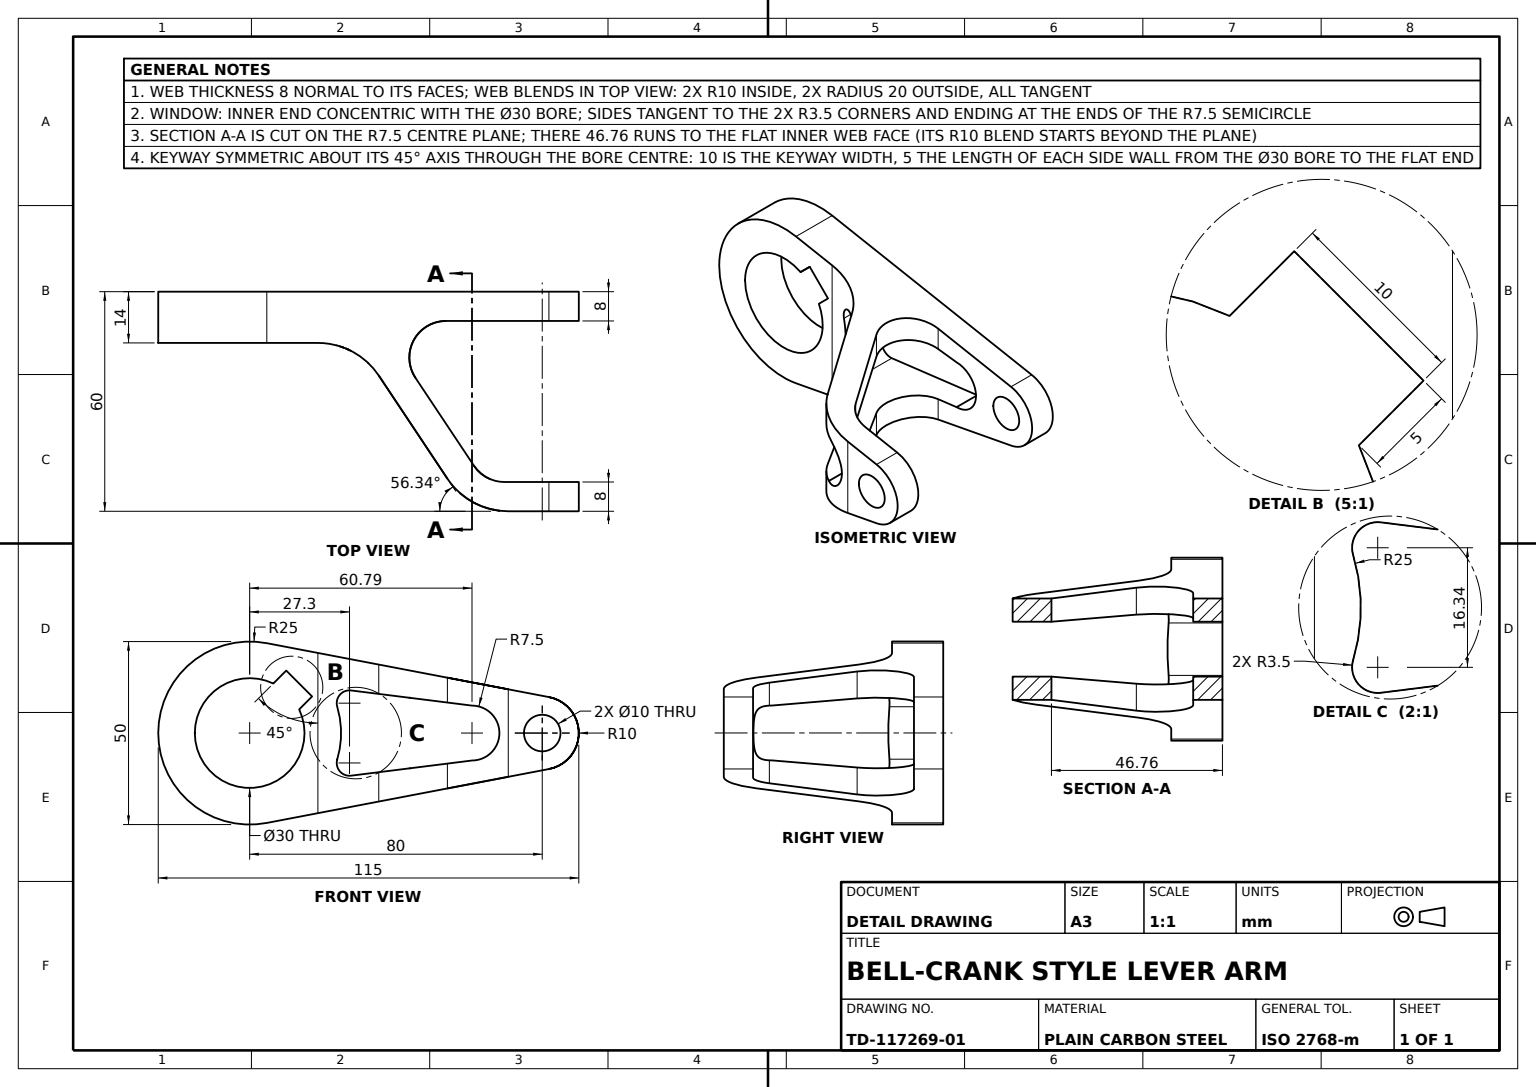
SolidWorks part; units mm, degrees
material "Plain Carbon Steel"
ref_plane "Front Plane" through (0, 0, 0) normal (0, 0, 1) x (1, 0, 0)
ref_plane "Top Plane" through (0, 0, 0) normal (0, 1, 0) x (1, 0, 0)
ref_plane "Right Plane" through (0, 0, 0) normal (1, 0, 0) x (0, 0, -1)
sketch "Lever Arm Profile Sketch" plane through (0, 0, 0) normal (0, 0, 1) x (1, 0, 0)
  line L0 (0, 48.8095) -> (0, -57.5397) construction
  line L1 (-106.9444, 0) -> (101.1905, 0) construction
  line L2 (81.8227, 9.8325) -> (4.6875, 24.5566)
  line L3 (81.8227, -9.8325) -> (4.6875, -24.5566)
  line L4 (60.7926, 7.5) -> (27.7394, 11.6416)
  line L5 (60.7926, -7.5) -> (27.7394, -11.6416)
  line L6 (0, 0) -> (39.4033, 39.4033) construction
  line L7 (10, 17.0711) -> (6.4645, 13.5355)
  line L8 (10, 17.0711) -> (17.0711, 10)
  line L9 (17.0711, 10) -> (13.5355, 6.4645)
  arc A0 (6.4645, 13.5355) -> (13.5355, 6.4645) centre (0, 0) ccw
  arc A1 (4.6875, 24.5566) -> (4.6875, -24.5566) centre (0, 0) ccw
  circle A2 centre (80, 0) radius 5
  arc A3 (81.8227, -9.8325) -> (81.8227, 9.8325) centre (80, 0) ccw
  arc A4 (60.7926, -7.5) -> (60.7926, 7.5) centre (60.7926, 0) ccw
  arc A5 (27.7394, 11.6416) -> (23.9511, 7.1655) centre (27.3043, 8.1687) ccw
  arc A6 (27.7394, -11.6416) -> (23.9511, -7.1655) centre (27.3043, -8.1687) cw
  arc A7 (23.9511, -7.1655) -> (23.9511, 7.1655) centre (0, 0) ccw
  point P28 (13.5355, 13.5355)
  dimension "D1" = 50
  dimension "D2" = 30
  dimension "D3" = 20
  dimension "D4" = 10
  dimension "D6" = 15
  dimension "D7" = 7
  dimension "D5" = 80
  dimension "D8" = 45
  dimension "D9" = 5
  dimension "D10" = 5
  dimension "D11" = 77.1351
  dimension "D12" = 77.1351
  dimension "D13" = 33.0532
extrude "Lever Arm Body" add sketch "Lever Arm Profile Sketch" along normal blind 60
sketch "Relief Cut Layout Sketch" plane through (0, 0, 0) normal (0, 1, 0) x (1, 0, 0)
  line L0 (0, 14.5595) -> (0, -50.2702) construction
  line L1 (-12.7585, -30) -> (100.8246, -30) construction
  line L2 (81.8227, 0) -> (4.6875, 0) construction
  dimension "D1" = 30
sketch "Relief Cut Profile Sketch" plane through (0, 0, 0) normal (0, 1, 0) x (1, 0, 0)
  line L0 (-25, -14) -> (18.6545, -14)
  line L1 (-25, 0) -> (-25, -60) construction
  line L2 (35.3007, -22.9137) -> (54.0635, -51.0863)
  line L3 (81.8227, -60) -> (4.6875, -60) construction
  line L4 (70.7097, -60) -> (90, -60)
  line L5 (90, -60) -> (90, -52)
  line L6 (90, -52) -> (69.6387, -52)
  line L7 (61.3156, -47.5431) -> (45.3317, -23.5431)
  line L9 (53.6548, -8) -> (90, -8)
  line L10 (90, -60) -> (90, 0) construction
  line L11 (90, -8) -> (90, 0)
  line L12 (90, 0) -> (-25, 0)
  line L13 (-25, 0) -> (-25, -14)
  line L14 (0, 14.5595) -> (0, -50.2702) construction
  line L15 (-25, -14) -> (-25, -60)
  line L16 (-25, -60) -> (90, -60)
  line L17 (90, -8) -> (90, -52)
  arc A0 (69.6387, -52) -> (61.3156, -47.5431) centre (69.6387, -42) cw
  arc A1 (53.6548, -8) -> (45.3317, -23.5431) centre (53.6548, -18) ccw
  arc A2 (18.6545, -14) -> (35.3007, -22.9137) centre (18.6545, -34) cw
  arc A3 (54.0635, -51.0863) -> (70.7097, -60) centre (70.7097, -40) ccw
  point P31 (60, -60)
  dimension "D6" = 10
  dimension "D7" = 20
  dimension "D8" = 10.031
  dimension "D1" = 8
  dimension "D2" = 8
  dimension "D3" = 14
  dimension "D4" = 8
  dimension "D5" = 60
extrude "Arm Relief Cut" cut sketch "Relief Cut Profile Sketch" against normal through all both and the other way through all contours A3 L2 A2 L0 L15 L16 | L9 A1 L7 A0 L6 L17
